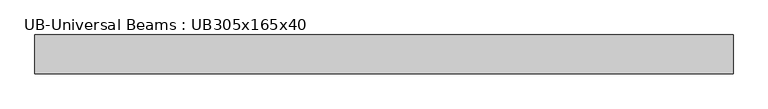
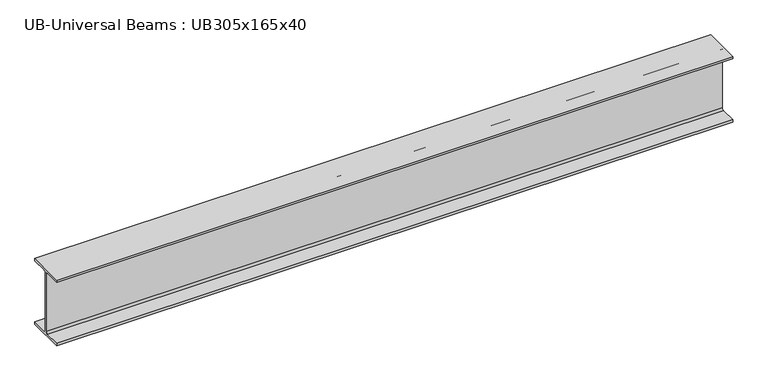
"""IFC4 building model written with IfcOpenShell, lengths in millimetres: beam geometry, UB-Universal Beams : UB305x165x40."""

from ifc_helpers import new_model, si_unit, point, frame, frame_2d, origin, place, context, project, spatial, polyline, circle_curve, trimmed, segment, composite_curve, outline, extrude, source, transform, mapped, element, save


def ub_universal_beams_ub305x165x40_3a463868(model_context):
    return source(origin(), model_context, "Body", "SweptSolid", [
        extrude(outline(composite_curve([segment(polyline([(82.5, -141.5), (82.5, -151.7), (-82.5, -151.7), (-82.5, -141.5), (-11.9, -141.5)]), True, "CONTINUOUS"), segment(trimmed(circle_curve(frame_2d((-11.9, -132.6)), 8.9), [point((-11.9, -141.5))], [point((-3.0, -132.6))], True, "CARTESIAN"), True, "CONTINUOUS"), segment(polyline([(-3.0, -132.6), (-3.0, 132.6)]), True, "CONTINUOUS"), segment(trimmed(circle_curve(frame_2d((-11.9, 132.6)), 8.9), [point((-3.0, 132.6))], [point((-11.9, 141.5))], True, "CARTESIAN"), True, "CONTINUOUS"), segment(polyline([(-11.9, 141.5), (-82.5, 141.5), (-82.5, 151.7), (82.5, 151.7), (82.5, 141.5), (11.9, 141.5)]), True, "CONTINUOUS"), segment(trimmed(circle_curve(frame_2d((11.9, 132.6)), 8.9), [point((11.9, 141.5))], [point((3.0, 132.6))], True, "CARTESIAN"), True, "CONTINUOUS"), segment(polyline([(3.0, 132.6), (3.0, -132.6)]), True, "CONTINUOUS"), segment(trimmed(circle_curve(frame_2d((11.9, -132.6)), 8.9), [point((3.0, -132.6))], [point((11.9, -141.5))], True, "CARTESIAN"), True, "CONTINUOUS"), segment(polyline([(11.9, -141.5), (82.5, -141.5)]), True, "CONTINUOUS")], self_intersect=False)), frame((-1535.35, 0.0, 0.0), z_axis=(1.0, 0.0, 0.0), x_axis=(0.0, 1.0, 0.0)), (0.0, 0.0, 1.0), 2958.0),
    ])


if __name__ == "__main__":
    model = new_model("IFC4")
    model_context = context("Model", 3, world=origin())
    ifc_project = project(units=[si_unit("LENGTHUNIT", "METRE", prefix="MILLI")], contexts=[model_context])
    site = spatial("IfcSite", under=ifc_project)
    building = spatial("IfcBuilding", under=site)
    placement = place(None, origin())
    ub_universal_beams_ub305x165x40_shape = ub_universal_beams_ub305x165x40_3a463868(model_context)
    element("IfcBeam", 1, ObjectType="UB-Universal Beams : UB305x165x40", at=placement, inside=building, context=model_context, shape_type="MappedRepresentation", body=[
        mapped(ub_universal_beams_ub305x165x40_shape, transform((0.0, 0.0, 0.0), x_axis=(1.0, 0.0, 0.0), y_axis=(0.0, 1.0, 0.0), z_axis=(0.0, 0.0, 1.0))),
    ])
    save(model, "model.ifc")

# Revit data of these elements
# Type "UB-Universal Beams : UB305x165x40"
#   Section Name Key = "UB305X165X40"
#   Width = 16.5 cm
#   Web Thickness = 0.6 cm
#   Web Fillet = 0.89 cm
#   Warping Constant = 164000.0 cm⁶
#   Torsional Moment of Inertia = 14.70 cm⁴
#   Section Area = 51.3 cm²
#   Plastic Modulus weak axis = 142.0 cm³
#   Plastic Modulus strong axis = 623.0 cm³
#   Nominal Weight = 40.2999 kgf/m
#   Moment of Inertia weak axis = 764.00 cm⁴
#   Moment of Inertia strong axis = 8503.00 cm⁴
#   Height = 30.34 cm
#   Flange Thickness = 1.02 cm
#   Elastic Modulus weak axis = 92.6 cm³
#   Elastic Modulus strong axis = 560.0 cm³
#   Centroid Vertical = 15.17 cm
#   Centroid Horizontal = 8.25 cm
#   Bolt Spacing = 9.0 cm
#   Length [instance default] = 1.5 m
#   Structural Material [instance default] = Metal - Steel 43-275
#   Type Comments = ""
#   Assembly Code = ""
# Element 1 (IfcBeam, "UB-Universal Beams : UB305x165x40")
#   Materials on its faces: "Metal - Steel 43-275"
# Materials
#   "Metal - Steel 43-275": class "Metal", colour RGB 247 247 247, transparency 0, Cost = 0
